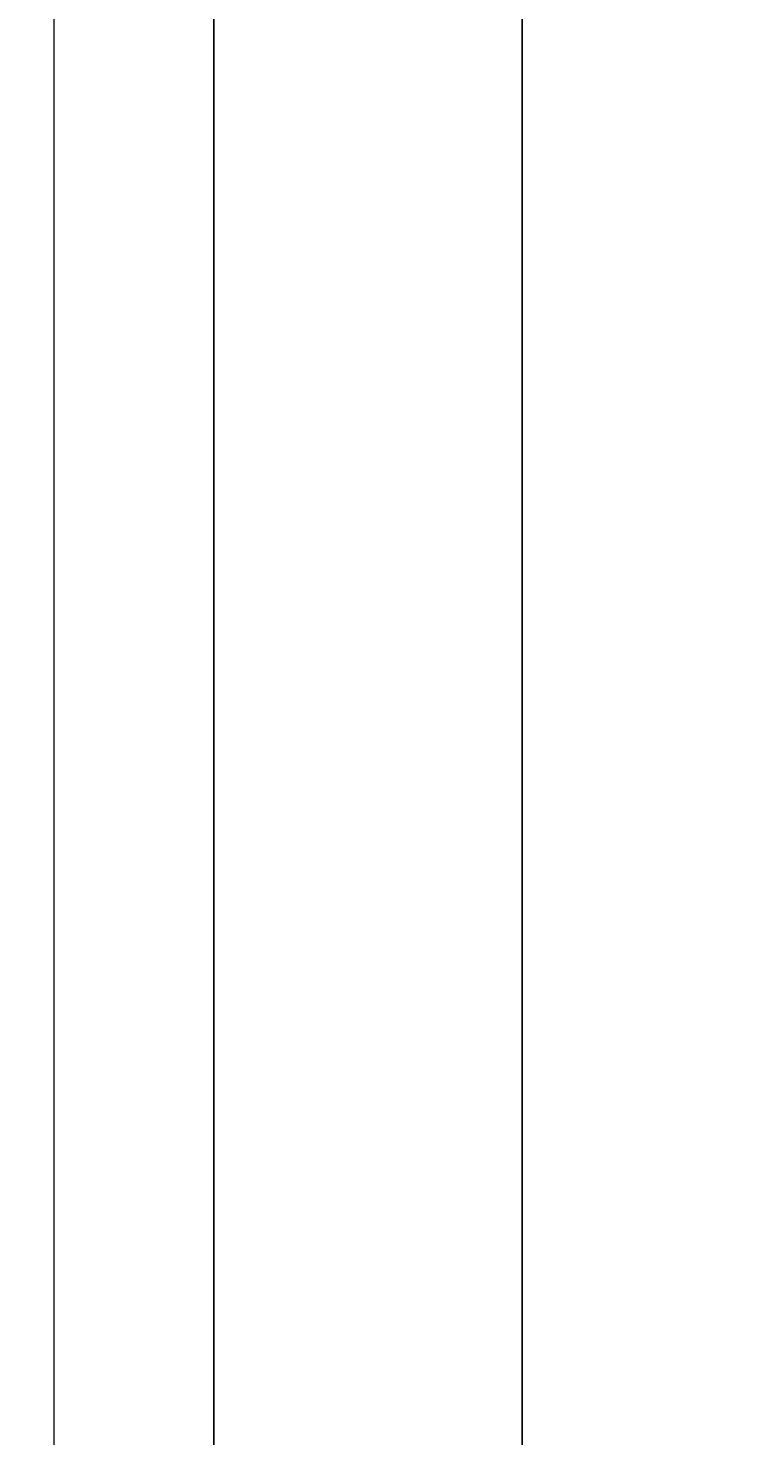
# Model space of a CAD drawing. Units: inches. Extents: x -46 to 1145, y -527 to 760.
# Tile 3 of 57: x 187 to 272, y -435 to -270. Entities that reach past the tile are written whole.
import ezdxf

# ---------------------------------------------------------------- set-up
doc = ezdxf.new("R2010")
doc.units = ezdxf.units.IN
doc.header["$MEASUREMENT"] = 0
doc.layers.add('A-ANNO-DIMS', color=2, linetype='Continuous', lineweight=18)
doc.layers.add('C-ROAD', color=9, linetype='Continuous', lineweight=18)
doc.styles.get("Standard").update_dxf_attribs({"font": 'arial.ttf'})
doc.dimstyles.get("Standard").update_dxf_attribs({"dimtxt": 0.18, "dimasz": 0.18, "dimexe": 0.18, "dimexo": 0.0625, "dimgap": 0.09, "dimtad": 0, "dimtih": 1, "dimtoh": 1, "dimdec": 0, "dimzin": 0, "dimdsep": 46, "dimlunit": 3, "dimtxsty": 'Standard', "dimcen": 0.09, "dimadec": 0, "dimazin": 0, "dimtfac": 1, "dimtdec": 0, "dimtofl": 0, "dimtmove": 0, "dimatfit": 3, "dimfxl": 1, "dimtolj": 1, "dimtzin": 0, "dimarcsym": 0})

# ---------------------------------------------------------------- blocks, each defined once
blk = doc.blocks.new('*D695')
at = {"layer": 'A-ANNO-DIMS', "color": 0, "lineweight": -2, "transparency": 16777216}
for p, q in [((208.27, 221.46), (208.27, -527.26)), ((244.27, 221.46), (244.27, -527.26)), ((208.45, -527.08), (226.05, -527.08)), ((244.09, -527.08), (226.49, -527.08))]:
    blk.add_line(p, q, dxfattribs=at)
at = {"layer": 'A-ANNO-DIMS', "color": 0, "transparency": 16777216}
for points in [[(208.45, -527.05), (208.45, -527.11), (208.27, -527.08)], [(244.09, -527.05), (244.09, -527.11), (244.27, -527.08)]]:
    blk.add_solid(points, dxfattribs=at)
at = {"layer": 'Defpoints', "color": 0, "transparency": 16777216}
for p in [(208.27, 221.52), (244.27, 221.52), (244.27, -527.08)]:
    blk.add_point(p, dxfattribs=at)
at = {"layer": 'A-ANNO-DIMS', "color": 0, "transparency": 16777216, "insert": (226.27, -527.08), "char_height": 0.18, "attachment_point": 5}
blk.add_mtext('\\A1;36', dxfattribs=at)
blk = doc.blocks.new('*D702')
at = {"layer": 'A-ANNO-DIMS', "color": 0, "lineweight": -2, "transparency": 16777216}
for p, q in [((189.63, -39.48), (1145.34, -39.48)), ((1145.16, -39.66), (1145.16, -249.3)), ((1145.16, -459.3), (1145.16, -249.66)), ((183.63, -459.48), (1145.34, -459.48))]:
    blk.add_line(p, q, dxfattribs=at)
at = {"layer": 'A-ANNO-DIMS', "color": 0, "transparency": 16777216}
for points in [[(1145.13, -39.66), (1145.19, -39.66), (1145.16, -39.48)], [(1145.13, -459.3), (1145.19, -459.3), (1145.16, -459.48)]]:
    blk.add_solid(points, dxfattribs=at)
at = {"layer": 'Defpoints', "color": 0, "transparency": 16777216}
for p in [(189.56, -39.48), (1145.16, -39.48), (183.56, -459.48)]:
    blk.add_point(p, dxfattribs=at)
at = {"layer": 'A-ANNO-DIMS', "color": 0, "transparency": 16777216, "insert": (1145.16, -249.48), "char_height": 0.18, "attachment_point": 5}
blk.add_mtext('\\A1;420', dxfattribs=at)

msp = doc.modelspace()

# ---------------------------------------------------------------- linework, layer by layer
at = {"layer": 'C-ROAD'}
msp.add_line((189.5637, 221.5176), (189.5637, -468.4824), dxfattribs=at)

# ---------------------------------------------------------------- dimensions: what is measured, and where the dimension line sits
at = {"layer": 'A-ANNO-DIMS'}
dim = msp.add_linear_dim(base=(244.2731, -527.0824), p1=(208.2731, 221.5176), p2=(244.2731, 221.5176), dimstyle='Standard', override={"dimdec": 0, "dimlfac": 1, "dimrnd": 0, "dimzin": 0, "dimdsep": 46, "dimlunit": 2}, dxfattribs=at)
dim.commit()
dim.dimension.update_dxf_attribs({"geometry": '*D695', "text_midpoint": (226.2731, -527.0824)})
dim = msp.add_linear_dim(base=(1145.1637, -39.4824), p1=(183.5637, -459.4824), p2=(189.5637, -39.4824), angle=90, dimstyle='Standard', override={"dimdec": 0, "dimlfac": 1, "dimrnd": 0, "dimzin": 0, "dimdsep": 46, "dimlunit": 2}, dxfattribs=at)
dim.commit()
dim.dimension.update_dxf_attribs({"geometry": '*D702', "text_midpoint": (1145.1637, -249.4824)})

doc.saveas('drawing.dxf')
